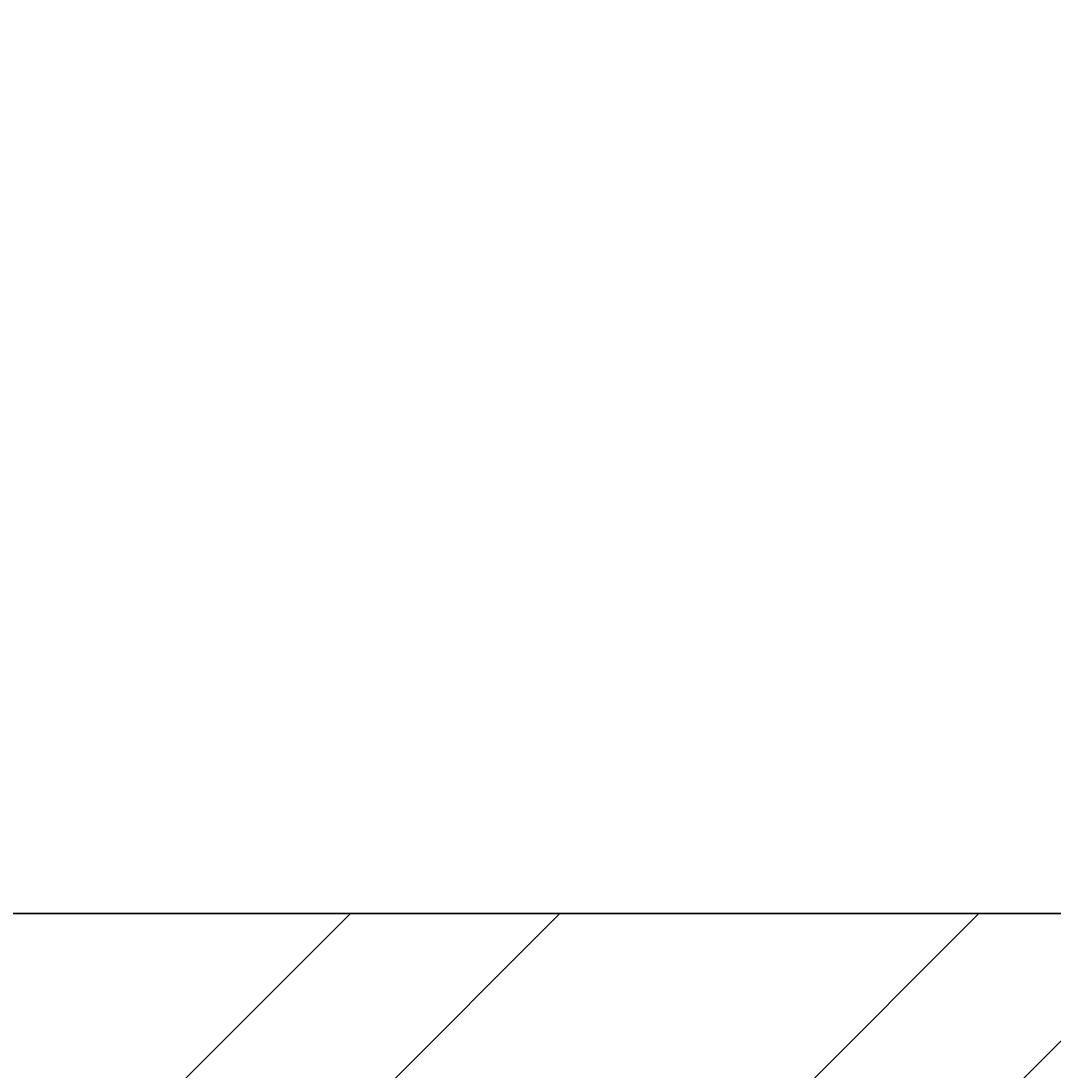
# Model space of a CAD drawing. Units: inches. Extents: x 1962 to 2771, y 1245 to 2660.
# Tile 39 of 114: x 2094.14 to 2116.25, y 2030.47 to 2052.97. Entities that reach past the tile are written whole.
import ezdxf

# ---------------------------------------------------------------- set-up
doc = ezdxf.new("R2010")
doc.units = ezdxf.units.IN
for name, color, linetype, lineweight in [('A-ANNO-DIMS', 2, 'Continuous', 18), ('A-WALL', 7, 'Continuous', 35), ('A-WALL-PATT', 252, 'Continuous', 13)]:
    doc.layers.add(name, color=color, linetype=linetype, lineweight=lineweight)
doc.styles.get("Standard").update_dxf_attribs({"font": 'arial.ttf'})
doc.dimstyles.get("Standard").update_dxf_attribs({"dimtxt": 0.18, "dimasz": 0.18, "dimexe": 0.18, "dimexo": 0.0625, "dimgap": 0.09, "dimtad": 0, "dimtih": 1, "dimtoh": 1, "dimdec": 4, "dimzin": 0, "dimdsep": 46, "dimtxsty": 'Standard', "dimcen": 0.09, "dimadec": 0, "dimazin": 0, "dimtfac": 1, "dimtdec": 4, "dimtofl": 0, "dimtmove": 0, "dimatfit": 3, "dimfxl": 1, "dimtolj": 1, "dimtzin": 0, "dimarcsym": 0})

# ---------------------------------------------------------------- blocks, each defined once
blk = doc.blocks.new('*D40')
at = {"layer": 'A-ANNO-DIMS', "color": 0, "lineweight": -2, "transparency": 16777216}
for p, q in [((2072.02, 2033.906), (2072.02, 2583.474)), ((2660.807, 2524.406), (2660.807, 2583.474)), ((2072.2, 2583.294), (2366.02, 2583.294)), ((2660.627, 2583.294), (2366.808, 2583.294))]:
    blk.add_line(p, q, dxfattribs=at)
at = {"layer": 'A-ANNO-DIMS', "color": 0, "transparency": 16777216}
for points in [[(2072.2, 2583.324), (2072.2, 2583.264), (2072.02, 2583.294)], [(2660.627, 2583.324), (2660.627, 2583.264), (2660.807, 2583.294)]]:
    blk.add_solid(points, dxfattribs=at)
at = {"layer": 'Defpoints', "color": 0, "transparency": 16777216}
for p in [(2660.807, 2583.294), (2660.807, 2524.344), (2072.02, 2033.844)]:
    blk.add_point(p, dxfattribs=at)
at = {"layer": 'A-ANNO-DIMS', "color": 0, "transparency": 16777216, "insert": (2366.414, 2583.294), "char_height": 0.18, "attachment_point": 5}
blk.add_mtext('\\A1;588.8', dxfattribs=at)

msp = doc.modelspace()

# ---------------------------------------------------------------- hatches: boundary and pattern name
at = {"layer": 'A-WALL-PATT'}
h = msp.add_hatch(dxfattribs=at)
h.set_pattern_fill('ANSI32', color=256)
h.paths.add_polyline_path([(2090.8074, 2467.3437), (2141.6481, 2467.3437), (2141.6481, 2469.5937), (2141.6481, 2471.8437), (2086.3074, 2471.8437), (2086.3074, 2422.5333), (2090.8074, 2422.5333)])
h.paths.add_polyline_path([(2282.7664, 2471.8437), (2204.8982, 2471.8437), (2204.8982, 2467.3437), (2234.8074, 2467.3437), (2234.8074, 2311.3437), (2228.7492, 2311.3437), (2228.7492, 2306.8437), (2234.8074, 2306.8437), (2331.9227, 2306.8437), (2331.9227, 2309.0937), (2331.9227, 2311.3437), (2239.3074, 2311.3437), (2239.3074, 2467.3437), (2282.7664, 2467.3437), (2282.7664, 2469.5937)])
h.paths.add_polyline_path([(2471.4531, 2519.8437), (2552.011, 2519.8437), (2564.3996, 2519.8437), (2564.3996, 2511.1389), (2568.8996, 2511.1389), (2568.8996, 2524.3437), (2466.9531, 2524.3437), (2466.9531, 2471.8437), (2450.0749, 2471.8437), (2446.4672, 2471.8437), (2446.4672, 2467.3437), (2450.0749, 2467.3437), (2475.9988, 2467.3437), (2475.9988, 2469.5937), (2475.9988, 2471.8437), (2471.4531, 2471.8437)])
h.paths.add_polyline_path([(2575.2231, 2469.5937), (2575.2231, 2471.8437), (2568.8996, 2471.8437), (2568.8996, 2487.1389), (2564.3996, 2487.1389), (2564.3996, 2471.8437), (2556.511, 2471.8437), (2499.2904, 2471.8437), (2499.2904, 2467.3437), (2507.8074, 2467.3437), (2507.8074, 2311.3437), (2414.863, 2311.3437), (2414.863, 2306.8437), (2512.3074, 2306.8437), (2517.0114, 2306.8437), (2517.0114, 2309.0937), (2517.0114, 2311.3437), (2512.3074, 2311.3437), (2512.3074, 2467.3437), (2575.2231, 2467.3437)])
h.paths.add_polyline_path([(2660.8074, 2471.8437), (2600.9602, 2471.8437), (2600.9602, 2467.3437), (2656.3074, 2467.3437), (2656.3074, 2432.5704), (2660.8074, 2432.5704)])
h.paths.add_polyline_path([(2660.8074, 2372.5704), (2656.3074, 2372.5704), (2656.3074, 2311.3437), (2600.276, 2311.3437), (2600.276, 2309.0937), (2600.276, 2306.8437), (2656.3074, 2306.8437), (2656.3074, 2296.2593), (2660.8074, 2296.2593)])
h.paths.add_polyline_path([(2572.3074, 2306.8437), (2577.1385, 2306.8437), (2577.1385, 2311.3437), (2551.082, 2311.3437), (2551.082, 2306.8437), (2567.8074, 2306.8437), (2567.8074, 2258.8437), (2540.0574, 2258.8437), (2540.0574, 2256.5937), (2540.0574, 2254.3437), (2567.8074, 2254.3437), (2656.3074, 2254.3437), (2656.3074, 2236.9085), (2660.8074, 2236.9085), (2660.8074, 2272.2593), (2656.3074, 2272.2593), (2656.3074, 2258.8437), (2572.3074, 2258.8437)])
h.paths.add_polyline_path([(2512.3074, 2254.3437), (2518.8716, 2254.3437), (2518.8716, 2256.5937), (2518.8716, 2258.8437), (2507.8074, 2258.8437), (2507.8074, 2177.8437), (2567.8074, 2177.8437), (2567.8074, 2172.9628), (2572.3074, 2172.9628), (2572.3074, 2177.8437), (2656.3074, 2177.8437), (2656.3074, 2166.4846), (2660.8074, 2166.4846), (2660.8074, 2200.9085), (2656.3074, 2200.9085), (2656.3074, 2182.3437), (2512.3074, 2182.3437)])
h.paths.add_polyline_path([(2656.3074, 2129.8437), (2572.3074, 2129.8437), (2572.3074, 2150.3044), (2570.0574, 2150.3044), (2567.8074, 2150.3044), (2567.8074, 2129.8437), (2507.8074, 2129.8437), (2507.8074, 2116.3027), (2510.0574, 2116.3027), (2512.3074, 2116.3027), (2512.3074, 2125.3437), (2567.8074, 2125.3437), (2572.3074, 2125.3437), (2656.3074, 2125.3437)])
h.paths.add_polyline_path([(2090.8074, 2362.5333), (2086.3074, 2362.5333), (2086.3074, 2298.6242), (2090.8074, 2298.6242), (2090.8074, 2306.8437), (2174.8074, 2306.8437), (2174.8074, 2286.4178), (2179.3074, 2286.4178), (2179.3074, 2306.8437), (2192.8641, 2306.8437), (2192.8641, 2309.0937), (2192.8641, 2311.3437), (2090.8074, 2311.3437)])
h.paths.add_polyline_path([(2209.156, 2258.8437), (2179.3074, 2258.8437), (2179.3074, 2263.2236), (2177.0574, 2263.2236), (2174.8074, 2263.2236), (2174.8074, 2258.8437), (2090.8074, 2258.8437), (2090.8074, 2274.6242), (2086.3074, 2274.6242), (2086.3074, 2238.2967), (2088.5574, 2238.2967), (2090.8074, 2238.2967), (2090.8074, 2254.3437), (2209.156, 2254.3437)])
h.paths.add_polyline_path([(2090.8074, 2177.8437), (2234.8074, 2177.8437), (2234.8074, 2173.1428), (2239.3074, 2173.1428), (2239.3074, 2258.8437), (2230.8442, 2258.8437), (2230.8442, 2256.5937), (2230.8442, 2254.3437), (2234.8074, 2254.3437), (2234.8074, 2182.3437), (2090.8074, 2182.3437), (2090.8074, 2202.2967), (2086.3074, 2202.2967), (2086.3074, 2140.0389), (2090.8074, 2140.0389)])
h.paths.add_polyline_path([(2090.8074, 2080.0389), (2086.3074, 2080.0389), (2086.3074, 2033.8437), (2090.8074, 2033.8437)], flags=17)
h.paths.add_polyline_path([(2244.9405, 2033.8437), (2239.3074, 2033.8437), (2239.3074, 2142.0665), (2237.2592, 2142.0665), (2234.8074, 2142.0665), (2234.8074, 2033.8437), (2090.8074, 2033.8437), (2076.5204, 2033.8437), (2072.0204, 2033.8437), (2072.0204, 2000.4493), (2076.5204, 2000.4493), (2076.5204, 2029.3437), (2090.8074, 2029.3437), (2244.9405, 2029.3437), (2244.9405, 2031.5937)])
h.paths.add_polyline_path([(2234.8074, 1933.3437), (2076.5204, 1933.3437), (2076.5204, 1952.4493), (2074.2704, 1952.4493), (2072.0204, 1952.4493), (2072.0204, 1933.3437), (2072.0204, 1928.8437), (2234.8074, 1928.8437)])
h.paths.add_polyline_path([(2090.8074, 1928.8437), (2086.3074, 1928.8437), (2086.3074, 1906.5013), (2090.8074, 1906.5013)])
h.paths.add_polyline_path([(2090.8074, 1846.5013), (2086.3074, 1846.5013), (2086.3074, 1769.9917), (2088.5574, 1769.9917), (2090.8074, 1769.9917), (2090.8074, 1780.3437), (2234.8074, 1780.3437), (2234.8074, 1708.3437), (2230.3764, 1708.3437), (2230.3764, 1703.8437), (2239.3074, 1703.8437), (2239.3074, 1792.6669), (2237.0574, 1792.6669), (2234.8074, 1792.6669), (2234.8074, 1784.8437), (2090.8074, 1784.8437)])
h.paths.add_polyline_path([(2239.3074, 1928.8437), (2244.9405, 1928.8437), (2244.9405, 1931.0937), (2244.9405, 1933.3437), (2234.8074, 1933.3437), (2234.8074, 1928.8437), (2234.8074, 1825.5949), (2239.3074, 1825.5949)])
h.paths.add_polyline_path([(2148.0425, 1649.0937), (2148.0425, 1651.3437), (2090.8074, 1651.3437), (2090.8074, 1646.8437), (2148.0425, 1646.8437)], flags=0)
h.paths.add_polyline_path([(2207.5601, 1708.3437), (2090.8074, 1708.3437), (2090.8074, 1703.8437), (2174.8074, 1703.8437), (2174.8074, 1651.3437), (2170.4457, 1651.3437), (2170.4457, 1646.8437), (2195.9924, 1646.8437), (2195.9924, 1649.0937), (2195.9924, 1651.3437), (2179.3074, 1651.3437), (2179.3074, 1703.8437), (2207.5601, 1703.8437), (2207.5601, 1706.0937)])
h.paths.add_polyline_path([(2090.8074, 1733.9917), (2086.3074, 1733.9917), (2086.3074, 1696.1032), (2088.5574, 1696.1032), (2090.8074, 1696.1032)])
h.paths.add_polyline_path([(2090.8074, 1672.1032), (2086.3074, 1672.1032), (2086.3074, 1600.3335), (2090.8074, 1600.3335)])
h.paths.add_polyline_path([(2090.8074, 1540.3335), (2086.3074, 1540.3335), (2086.3074, 1486.3437), (2139.6766, 1486.3437), (2139.6766, 1490.8437), (2090.8074, 1490.8437)])
h.paths.add_polyline_path([(2302.3876, 1490.8437), (2239.3074, 1490.8437), (2239.3074, 1646.8437), (2335.9994, 1646.8437), (2335.9994, 1651.3437), (2229.884, 1651.3437), (2229.884, 1646.8437), (2234.8074, 1646.8437), (2234.8074, 1490.8437), (2202.7103, 1490.8437), (2202.7103, 1488.5937), (2202.7103, 1486.3437), (2275.0699, 1486.3437), (2275.0699, 1475.772), (2279.5699, 1475.772), (2279.5699, 1486.3437), (2302.3876, 1486.3437)])
h.paths.add_polyline_path([(2279.5699, 1451.772), (2275.0699, 1451.772), (2275.0699, 1438.3437), (2174.8074, 1438.3437), (2174.8074, 1486.3437), (2179.7922, 1486.3437), (2179.7922, 1490.8437), (2163.3585, 1490.8437), (2163.3585, 1488.5937), (2163.3585, 1486.3437), (2170.3074, 1486.3437), (2170.3074, 1433.8437), (2279.5699, 1433.8437)])
h.paths.add_polyline_path([(2427.2363, 1490.8437), (2375.8074, 1490.8437), (2375.8074, 1646.8437), (2381.6401, 1646.8437), (2381.6401, 1651.3437), (2365.887, 1651.3437), (2365.887, 1649.0937), (2365.887, 1646.8437), (2371.3074, 1646.8437), (2371.3074, 1490.8437), (2327.5627, 1490.8437), (2327.5627, 1488.5937), (2327.5627, 1486.3437), (2371.3074, 1486.3437), (2371.3074, 1433.8437), (2375.8074, 1433.8437), (2375.8074, 1486.3437), (2427.2363, 1486.3437)])
h.paths.add_polyline_path([(2512.3074, 1646.8437), (2519.4351, 1646.8437), (2519.4351, 1649.0937), (2519.4351, 1651.3437), (2507.8074, 1651.3437), (2416.0063, 1651.3437), (2416.0063, 1649.0937), (2416.0063, 1646.8437), (2507.8074, 1646.8437), (2507.8074, 1490.8437), (2497.0532, 1490.8437), (2497.0532, 1488.5937), (2497.0532, 1486.3437), (2574.9344, 1486.3437), (2574.9344, 1476.0181), (2579.4344, 1476.0181), (2579.4344, 1486.3437), (2584.4872, 1486.3437), (2584.3074, 1490.8437), (2512.3074, 1490.8437)])
h.paths.add_polyline_path([(2470.5091, 1486.3437), (2473.9767, 1486.3437), (2473.9767, 1490.8437), (2449.6605, 1490.8437), (2449.6605, 1488.5937), (2449.6605, 1486.3437), (2466.0091, 1486.3437), (2466.0091, 1433.8437), (2470.5091, 1433.8437), (2579.4344, 1433.8437), (2579.4344, 1452.0181), (2574.9344, 1452.0181), (2574.9344, 1438.3437), (2554.5091, 1438.3437), (2470.5091, 1438.3437)])
h.paths.add_polyline_path([(2656.3074, 1490.8437), (2611.86, 1490.8437), (2611.86, 1486.3437), (2656.3074, 1486.3437)])
h.paths.add_polyline_path([(2660.8074, 1532.7007), (2658.5574, 1532.7007), (2656.3074, 1532.7007), (2656.3074, 1486.3437), (2660.8074, 1486.3437)])
h.paths.add_polyline_path([(2660.8074, 1664.9663), (2656.3074, 1664.9663), (2656.3074, 1651.3437), (2602.2313, 1651.3437), (2602.2313, 1646.8437), (2656.3074, 1646.8437), (2656.3074, 1592.7007), (2660.8074, 1592.7007)])
h.paths.add_polyline_path([(2660.8074, 1724.5221), (2656.3074, 1724.5221), (2656.3074, 1703.8437), (2542.4725, 1703.8437), (2542.4725, 1699.3437), (2567.8074, 1699.3437), (2567.8074, 1651.3437), (2552.7766, 1651.3437), (2552.7766, 1649.0937), (2552.7766, 1646.8437), (2577.2878, 1646.8437), (2577.2878, 1649.0937), (2577.2878, 1651.3437), (2572.3074, 1651.3437), (2572.3074, 1699.3437), (2656.3074, 1699.3437), (2656.3074, 1688.9663), (2660.8074, 1688.9663)])
h.paths.add_polyline_path([(2660.8074, 1880.6524), (2656.3074, 1880.6524), (2656.3074, 1832.8437), (2512.3074, 1832.8437), (2512.3074, 1837.8959), (2507.8074, 1837.8959), (2507.8074, 1828.3437), (2567.8074, 1828.3437), (2567.8074, 1804.3437), (2572.3074, 1804.3437), (2572.3074, 1828.3437), (2656.3074, 1828.3437), (2656.3074, 1818.6778), (2660.8074, 1818.6778)])
h.paths.add_polyline_path([(2660.8074, 1794.6778), (2656.3074, 1794.6778), (2656.3074, 1780.3437), (2572.3074, 1780.3437), (2572.3074, 1783.0303), (2570.0574, 1783.0303), (2567.8074, 1783.0303), (2567.8074, 1780.3437), (2507.8074, 1780.3437), (2507.8074, 1699.3437), (2517.8858, 1699.3437), (2517.8858, 1701.5937), (2517.8858, 1703.8437), (2512.3074, 1703.8437), (2512.3074, 1775.8437), (2656.3074, 1775.8437), (2656.3074, 1760.5221), (2660.8074, 1760.5221)])
h.paths.add_polyline_path([(2660.8074, 1981.3437), (2660.8074, 2020.2808), (2658.5574, 2020.2808), (2656.3074, 2020.2808), (2656.3074, 1981.3437), (2512.3074, 1981.3437), (2512.3074, 2086.6996), (2507.8074, 2086.6996), (2507.8074, 1981.3437), (2375.8074, 1981.3437), (2375.8074, 1986.8505), (2373.5574, 1986.8505), (2371.3074, 1986.8505), (2371.3074, 1973.2607), (2375.8074, 1973.2607), (2375.8074, 1976.8437), (2507.8074, 1976.8437), (2507.8074, 1865.4281), (2510.0574, 1865.4281), (2512.3074, 1865.4281), (2512.3074, 1976.8437), (2660.8074, 1976.8437)])
h.paths.add_polyline_path([(2375.8074, 1940.297), (2373.5574, 1940.297), (2371.3074, 1940.297), (2371.3074, 1933.3437), (2278.4434, 1933.3437), (2278.4434, 1928.8437), (2371.3074, 1928.8437), (2371.3074, 1651.3437), (2375.8074, 1651.3437)])
h.paths.add_polyline_path([(2660.8074, 1976.8437), (2656.3074, 1976.8437), (2656.3074, 1940.6524), (2660.8074, 1940.6524)], flags=17)
h.paths.add_polyline_path([(2660.8074, 2142.4846), (2656.3074, 2142.4846), (2656.3074, 2080.2808), (2660.8074, 2080.2808)])
h.paths.add_polyline_path([(2381.4189, 2311.3437), (2375.8074, 2311.3437), (2375.8074, 2467.3437), (2424.7242, 2467.3437), (2424.7242, 2469.5937), (2424.7242, 2471.8437), (2375.8074, 2471.8437), (2375.8074, 2524.3437), (2371.3074, 2524.3437), (2371.3074, 2471.8437), (2307.2097, 2471.8437), (2307.2097, 2467.3437), (2371.3074, 2467.3437), (2371.3074, 2311.3437), (2366.8901, 2311.3437), (2366.8901, 2306.8437), (2371.3074, 2306.8437), (2371.3074, 2033.8437), (2279.6589, 2033.8437), (2279.6589, 2029.3437), (2371.3074, 2029.3437), (2371.3074, 2014.2598), (2375.8074, 2014.2598), (2375.8074, 2306.8437), (2381.4189, 2306.8437)])
h.paths.add_polyline_path([(2263.3074, 2524.3437), (2170.3074, 2524.3437), (2170.3074, 2519.8437), (2170.3074, 2471.8437), (2165.0312, 2471.8437), (2165.0312, 2467.3437), (2179.6721, 2467.3437), (2179.6721, 2469.5161), (2179.6721, 2471.8437), (2174.8074, 2471.8437), (2174.8074, 2519.8437), (2258.8074, 2519.8437), (2258.8074, 2511.6436), (2263.3074, 2511.6436)])
h.paths.add_polyline_path([(2245.0232, 1361.4123), (2492.9468, 1361.4123), (2492.9468, 1398.505), (2245.0232, 1398.505)], flags=9)
h.paths.add_polyline_path([(2388.1434, 2086.6936), (2425.0704, 2086.6936), (2425.0704, 2105.3509), (2388.1434, 2105.3509)], flags=9)
h.paths.add_polyline_path([(2404.922, 2242.6744), (2445.7337, 2242.6744), (2445.7337, 2261.3318), (2404.922, 2261.3318)], flags=9)
h.paths.add_polyline_path([(2269.4107, 2156.7935), (2306.3378, 2156.7935), (2306.3378, 2175.4508), (2269.4107, 2175.4508)], flags=9)
h.paths.add_polyline_path([(2269.3277, 2233.4343), (2306.2547, 2233.4343), (2306.2547, 2252.0917), (2269.3277, 2252.0917)], flags=9)
h.paths.add_polyline_path([(2431.6052, 2320.6922), (2470.4456, 2320.6922), (2470.4456, 2339.3495), (2431.6052, 2339.3495)], flags=25)
h.paths.add_polyline_path([(2249.6902, 2315.7608), (2288.5306, 2315.7608), (2288.5306, 2334.4182), (2249.6902, 2334.4182)], flags=25)
h.paths.add_polyline_path([(2096.9301, 2314.3181), (2135.7704, 2314.3181), (2135.7704, 2332.9755), (2096.9301, 2332.9755)], flags=25)
h.paths.add_polyline_path([(2134.3475, 2285.7089), (2161.4655, 2285.7089), (2161.4655, 2304.3662), (2134.3475, 2304.3662)], flags=9)
h.paths.add_polyline_path([(2126.5155, 2209.4076), (2159.9227, 2209.4076), (2159.9227, 2228.065), (2126.5155, 2228.065)], flags=25)
h.paths.add_polyline_path([(2110.5753, 2141.5299), (2149.4157, 2141.5299), (2149.4157, 2160.1872), (2110.5753, 2160.1872)], flags=25)
h.paths.add_polyline_path([(2249.8618, 1968.3317), (2286.3966, 1968.3317), (2286.3966, 1986.989), (2249.8618, 1986.989)], flags=9)
h.paths.add_polyline_path([(2395.9507, 1777.0051), (2436.7624, 1777.0051), (2436.7624, 1795.6625), (2395.9507, 1795.6625)], flags=9)
h.paths.add_polyline_path([(2398.5259, 1888.5651), (2435.0062, 1888.5651), (2435.0062, 1907.2224), (2398.5259, 1907.2224)], flags=25)
h.paths.add_polyline_path([(2259.3506, 1728.3559), (2296.2776, 1728.3559), (2296.2776, 1747.0132), (2259.3506, 1747.0132)], flags=9)
h.paths.add_polyline_path([(2271.3698, 1845.268), (2308.2968, 1845.268), (2308.2968, 1863.9253), (2271.3698, 1863.9253)], flags=9)
h.paths.add_polyline_path([(2120.9355, 1786.3027), (2159.7759, 1786.3027), (2159.7759, 1804.9601), (2120.9355, 1804.9601)], flags=25)
h.paths.add_polyline_path([(2121.3164, 1732.1043), (2154.7236, 1732.1043), (2154.7236, 1750.7616), (2121.3164, 1750.7616)], flags=25)
h.paths.add_polyline_path([(2118.3706, 1678.8997), (2147.5282, 1678.8997), (2147.5282, 1697.557), (2118.3706, 1697.557)], flags=25)
h.paths.add_polyline_path([(2385.9227, 1493.557), (2424.763, 1493.557), (2424.763, 1512.2143), (2385.9227, 1512.2143)], flags=25)
h.paths.add_polyline_path([(2248.7058, 1500.0256), (2287.5462, 1500.0256), (2287.5462, 1518.6829), (2248.7058, 1518.6829)], flags=25)
h.paths.add_polyline_path([(2104.1669, 1617.3771), (2143.0073, 1617.3771), (2143.0073, 1636.0344), (2104.1669, 1636.0344)], flags=9)
h.paths.add_polyline_path([(2096.0714, 1447.8824), (2137.3845, 1447.8824), (2137.3845, 1458.1859), (2096.0714, 1458.1859)], flags=9)
h.paths.add_polyline_path([(2180.6114, 1440.325), (2209.7689, 1440.325), (2209.7689, 1458.9823), (2180.6114, 1458.9823)], flags=25)
h.paths.add_polyline_path([(2316.1698, 1447.9637), (2357.4829, 1447.9637), (2357.4829, 1458.2673), (2316.1698, 1458.2673)], flags=9)
h.paths.add_polyline_path([(2397.6187, 1447.9637), (2438.9318, 1447.9637), (2438.9318, 1458.2673), (2397.6187, 1458.2673)], flags=9)
h.paths.add_polyline_path([(2473.0778, 1439.5953), (2502.2354, 1439.5953), (2502.2354, 1458.2527), (2473.0778, 1458.2527)], flags=25)
h.paths.add_polyline_path([(2589.7027, 1447.8819), (2631.0158, 1447.8819), (2631.0158, 1458.1855), (2589.7027, 1458.1855)], flags=9)
h.paths.add_polyline_path([(2522.4009, 1497.5285), (2561.2413, 1497.5285), (2561.2413, 1516.1859), (2522.4009, 1516.1859)], flags=25)
h.paths.add_polyline_path([(2579.6565, 1671.3482), (2608.8141, 1671.3482), (2608.8141, 1690.0056), (2579.6565, 1690.0056)], flags=25)
h.paths.add_polyline_path([(2544.7038, 1725.5064), (2578.1111, 1725.5064), (2578.1111, 1744.1637), (2544.7038, 1744.1637)], flags=25)
h.paths.add_polyline_path([(2578.1191, 1807.472), (2607.2766, 1807.472), (2607.2766, 1826.1293), (2578.1191, 1826.1293)], flags=25)
h.paths.add_polyline_path([(2595.0614, 1835.1839), (2633.9018, 1835.1839), (2633.9018, 1853.8413), (2595.0614, 1853.8413)], flags=25)
h.paths.add_polyline_path([(2567.0097, 2097.7035), (2605.8501, 2097.7035), (2605.8501, 2116.3609), (2567.0097, 2116.3609)], flags=9)
h.paths.add_polyline_path([(2586.644, 2134.6454), (2615.8015, 2134.6454), (2615.8015, 2153.3027), (2586.644, 2153.3027)], flags=9)
h.paths.add_polyline_path([(2544.6185, 2212.6783), (2578.0258, 2212.6783), (2578.0258, 2231.3356), (2544.6185, 2231.3356)], flags=25)
h.paths.add_polyline_path([(2577.0273, 2256.9023), (2606.1849, 2256.9023), (2606.1849, 2275.5597), (2577.0273, 2275.5597)], flags=24)
h.paths.add_polyline_path([(2605.2683, 2315.2821), (2644.1087, 2315.2821), (2644.1087, 2333.9395), (2605.2683, 2333.9395)], flags=25)
h.paths.add_polyline_path([(2583.1244, 2496.1815), (2624.4375, 2496.1815), (2624.4375, 2506.4851), (2583.1244, 2506.4851)], flags=9)
h.paths.add_polyline_path([(2474.761, 2497.0823), (2503.9185, 2497.0823), (2503.9185, 2515.7397), (2474.761, 2515.7397)], flags=25)
h.paths.add_polyline_path([(2387.5787, 2494.2563), (2428.902, 2494.2563), (2428.902, 2504.5598), (2387.5787, 2504.5598)], flags=9)
h.paths.add_polyline_path([(2300.1657, 2500.1564), (2341.4788, 2500.1564), (2341.4788, 2510.46), (2300.1657, 2510.46)], flags=25)
h.paths.add_polyline_path([(2176.8589, 2497.5843), (2206.0165, 2497.5843), (2206.0165, 2516.2416), (2176.8589, 2516.2416)], flags=25)
h.paths.add_polyline_path([(2097.4668, 2494.9762), (2138.7799, 2494.9762), (2138.7799, 2505.2798), (2097.4668, 2505.2798)], flags=9)

# ---------------------------------------------------------------- linework, layer by layer
at = {"layer": 'A-WALL'}
msp.add_line((2090.8074, 2033.8437), (2234.8074, 2033.8437), dxfattribs=at)

# ---------------------------------------------------------------- dimensions: what is measured, and where the dimension line sits
at = {"layer": 'A-ANNO-DIMS'}
dim = msp.add_linear_dim(base=(2660.8074, 2583.2937), p1=(2072.0204, 2033.8437), p2=(2660.8074, 2524.3437), dimstyle='Standard', override={"dimdec": 1, "dimlfac": 1, "dimrnd": 0, "dimzin": 0, "dimdsep": 46, "dimlunit": 2}, dxfattribs=at)
dim.commit()
dim.dimension.update_dxf_attribs({"geometry": '*D40', "text_midpoint": (2366.4139, 2583.2937)})

doc.saveas('drawing.dxf')
